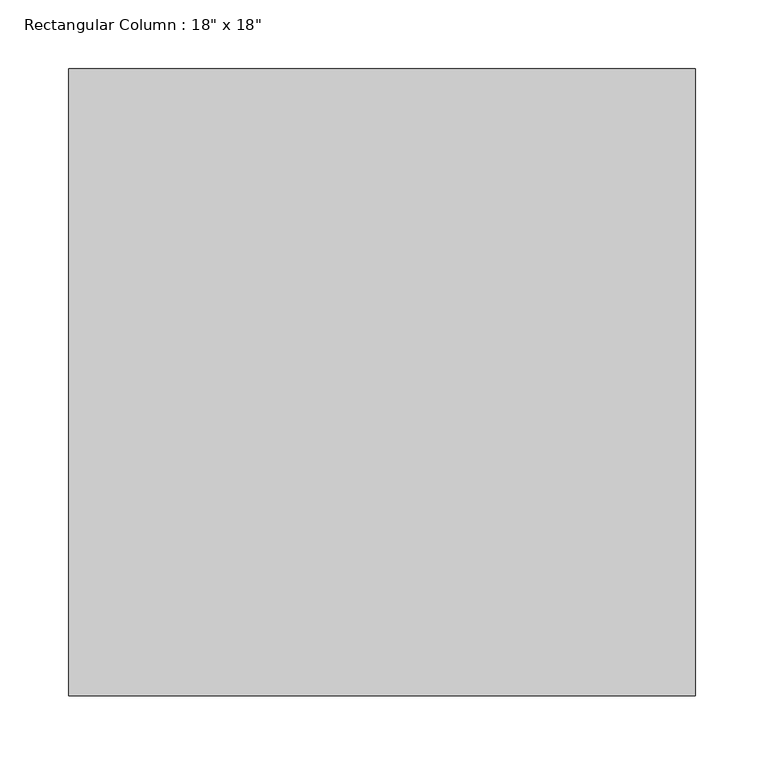
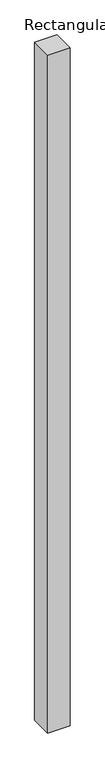
"""IFC4 building model written with IfcOpenShell, lengths in millimetres: column geometry."""

from ifc_helpers import new_model, si_unit, origin, origin_with_axes, place, context, project, spatial, polyline, outline, extrude, source, transform, mapped, element, save


def column_59a13550(model_context):
    return source(origin(), model_context, "Body", "SweptSolid", [
        extrude(outline(polyline([(228.6, 228.6), (228.6, -228.6), (-228.6, -228.6), (-228.6, 228.6), (228.6, 228.6)])), origin_with_axes(), (0.0, 0.0, 1.0), 14630.4),
    ])


if __name__ == "__main__":
    model = new_model("IFC4")
    model_context = context("Model", 3, world=origin())
    ifc_project = project(units=[si_unit("LENGTHUNIT", "METRE", prefix="MILLI")], contexts=[model_context])
    site = spatial("IfcSite", under=ifc_project)
    building = spatial("IfcBuilding", under=site)
    placement = place(None, origin())
    column_shape = column_59a13550(model_context)
    element("IfcColumn", 1, ObjectType="Rectangular Column : 18\" x 18\"", at=placement, inside=building, context=model_context, shape_type="MappedRepresentation", body=[
        mapped(column_shape, transform((0.0, 0.0, 0.0), x_axis=(1.0, 0.0, 0.0), y_axis=(0.0, 1.0, 0.0), z_axis=(0.0, 0.0, 1.0))),
    ])
    save(model, "model.ifc")

# Revit data of these elements
# Type "Rectangular Column : 18\" x 18\""
#   Assembly Code = "B1010200"
#   Depth = 1' - 6"
#   Offset Base = 0' - 0"
#   Offset Top = 0' - 0"
#   Width = 1' - 6"
#   Material = none
